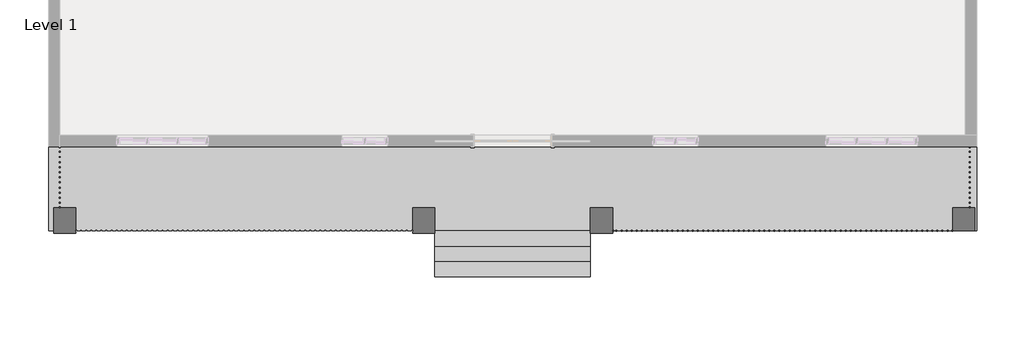
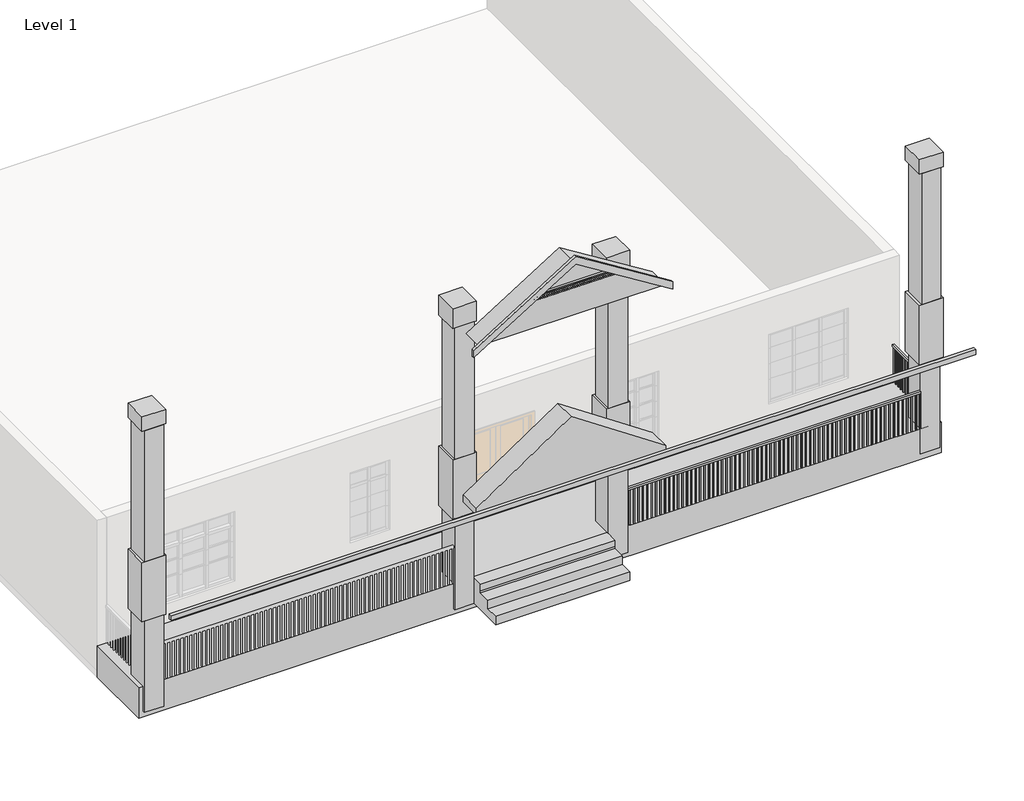
# One storey, part 3 of 3: 2 railings, 1 proxy.
"""IFC4 building model written with IfcOpenShell, lengths in millimetres."""

from ifc_helpers import new_model, si_unit, frame, origin, place, context, project, spatial, polyline, outline, extrude, transform, mapped, element, save
from components import generic_models_1_generic_models_1_befc9ee0

model = new_model("IFC4")

# Units and contexts
model_context = context("Model", 3, world=origin())
ifc_project = project(units=[si_unit("LENGTHUNIT", "METRE", prefix="MILLI")], contexts=[model_context])

# Site, building, storey
site = spatial("IfcSite", under=ifc_project)
building = spatial("IfcBuilding", under=site)
storey = spatial("IfcBuildingStorey", under=building, Name="Level 1", Elevation=0.0)

# Proxy
placement = place(None, origin())
generic_models_1_generic_models_1_shape = generic_models_1_generic_models_1_befc9ee0(model_context)
element("IfcBuildingElementProxy", 1, Name="Generic Models 1 : Generic Models 1", ObjectType="Generic Models 1 : Generic Models 1", at=placement, inside=storey, context=model_context, shape_type="MappedRepresentation", body=[
    mapped(generic_models_1_generic_models_1_shape, transform((0.0, 0.0, 0.0), x_axis=(1.0, 0.0, 0.0), y_axis=(0.0, 1.0, 0.0), z_axis=(0.0, 0.0, 1.0))),
])

# Railings
element("IfcRailing", 2, ObjectType="Handrail - Rectangular", at=placement, inside=storey, context=model_context, shape_type="SweptSolid", body=[
    extrude(outline(polyline([(8263.5579341, -8749.7902135), (8263.5579341, -8800.5902135), (1481.7579341, -8800.5902135), (1481.7579341, -8749.7902135), (8263.5579341, -8749.7902135)])), frame((0.0, 0.0, 1473.2), z_axis=(0.0, 0.0, 1.0), x_axis=(1.0, 0.0, 0.0)), (0.0, 0.0, 1.0), 50.8),
    extrude(outline(polyline([(1567.4829341, -8765.6652135), (1567.4829341, -8784.7152135), (1548.4329341, -8784.7152135), (1548.4329341, -8765.6652135), (1567.4829341, -8765.6652135)])), frame((0.0, 0.0, 609.6), z_axis=(0.0, 0.0, 1.0), x_axis=(1.0, 0.0, 0.0)), (0.0, 0.0, 1.0), 863.6),
    extrude(outline(polyline([(1669.0829341, -8765.6652135), (1669.0829341, -8784.7152135), (1650.0329341, -8784.7152135), (1650.0329341, -8765.6652135), (1669.0829341, -8765.6652135)])), frame((0.0, 0.0, 609.6), z_axis=(0.0, 0.0, 1.0), x_axis=(1.0, 0.0, 0.0)), (0.0, 0.0, 1.0), 863.6),
    extrude(outline(polyline([(1770.6829341, -8765.6652135), (1770.6829341, -8784.7152135), (1751.6329341, -8784.7152135), (1751.6329341, -8765.6652135), (1770.6829341, -8765.6652135)])), frame((0.0, 0.0, 609.6), z_axis=(0.0, 0.0, 1.0), x_axis=(1.0, 0.0, 0.0)), (0.0, 0.0, 1.0), 863.6),
    extrude(outline(polyline([(1872.2829341, -8765.6652135), (1872.2829341, -8784.7152135), (1853.2329341, -8784.7152135), (1853.2329341, -8765.6652135), (1872.2829341, -8765.6652135)])), frame((0.0, 0.0, 609.6), z_axis=(0.0, 0.0, 1.0), x_axis=(1.0, 0.0, 0.0)), (0.0, 0.0, 1.0), 863.6),
    extrude(outline(polyline([(1973.8829341, -8765.6652135), (1973.8829341, -8784.7152135), (1954.8329341, -8784.7152135), (1954.8329341, -8765.6652135), (1973.8829341, -8765.6652135)])), frame((0.0, 0.0, 609.6), z_axis=(0.0, 0.0, 1.0), x_axis=(1.0, 0.0, 0.0)), (0.0, 0.0, 1.0), 863.6),
    extrude(outline(polyline([(2075.4829341, -8765.6652135), (2075.4829341, -8784.7152135), (2056.4329341, -8784.7152135), (2056.4329341, -8765.6652135), (2075.4829341, -8765.6652135)])), frame((0.0, 0.0, 609.6), z_axis=(0.0, 0.0, 1.0), x_axis=(1.0, 0.0, 0.0)), (0.0, 0.0, 1.0), 863.6),
    extrude(outline(polyline([(2177.0829341, -8765.6652135), (2177.0829341, -8784.7152135), (2158.0329341, -8784.7152135), (2158.0329341, -8765.6652135), (2177.0829341, -8765.6652135)])), frame((0.0, 0.0, 609.6), z_axis=(0.0, 0.0, 1.0), x_axis=(1.0, 0.0, 0.0)), (0.0, 0.0, 1.0), 863.6),
    extrude(outline(polyline([(2278.6829341, -8765.6652135), (2278.6829341, -8784.7152135), (2259.6329341, -8784.7152135), (2259.6329341, -8765.6652135), (2278.6829341, -8765.6652135)])), frame((0.0, 0.0, 609.6), z_axis=(0.0, 0.0, 1.0), x_axis=(1.0, 0.0, 0.0)), (0.0, 0.0, 1.0), 863.6),
    extrude(outline(polyline([(2380.2829341, -8765.6652135), (2380.2829341, -8784.7152135), (2361.2329341, -8784.7152135), (2361.2329341, -8765.6652135), (2380.2829341, -8765.6652135)])), frame((0.0, 0.0, 609.6), z_axis=(0.0, 0.0, 1.0), x_axis=(1.0, 0.0, 0.0)), (0.0, 0.0, 1.0), 863.6),
    extrude(outline(polyline([(2481.8829341, -8765.6652135), (2481.8829341, -8784.7152135), (2462.8329341, -8784.7152135), (2462.8329341, -8765.6652135), (2481.8829341, -8765.6652135)])), frame((0.0, 0.0, 609.6), z_axis=(0.0, 0.0, 1.0), x_axis=(1.0, 0.0, 0.0)), (0.0, 0.0, 1.0), 863.6),
    extrude(outline(polyline([(2583.4829341, -8765.6652135), (2583.4829341, -8784.7152135), (2564.4329341, -8784.7152135), (2564.4329341, -8765.6652135), (2583.4829341, -8765.6652135)])), frame((0.0, 0.0, 609.6), z_axis=(0.0, 0.0, 1.0), x_axis=(1.0, 0.0, 0.0)), (0.0, 0.0, 1.0), 863.6),
    extrude(outline(polyline([(2685.0829341, -8765.6652135), (2685.0829341, -8784.7152135), (2666.0329341, -8784.7152135), (2666.0329341, -8765.6652135), (2685.0829341, -8765.6652135)])), frame((0.0, 0.0, 609.6), z_axis=(0.0, 0.0, 1.0), x_axis=(1.0, 0.0, 0.0)), (0.0, 0.0, 1.0), 863.6),
    extrude(outline(polyline([(2786.6829341, -8765.6652135), (2786.6829341, -8784.7152135), (2767.6329341, -8784.7152135), (2767.6329341, -8765.6652135), (2786.6829341, -8765.6652135)])), frame((0.0, 0.0, 609.6), z_axis=(0.0, 0.0, 1.0), x_axis=(1.0, 0.0, 0.0)), (0.0, 0.0, 1.0), 863.6),
    extrude(outline(polyline([(2888.2829341, -8765.6652135), (2888.2829341, -8784.7152135), (2869.2329341, -8784.7152135), (2869.2329341, -8765.6652135), (2888.2829341, -8765.6652135)])), frame((0.0, 0.0, 609.6), z_axis=(0.0, 0.0, 1.0), x_axis=(1.0, 0.0, 0.0)), (0.0, 0.0, 1.0), 863.6),
    extrude(outline(polyline([(2989.8829341, -8765.6652135), (2989.8829341, -8784.7152135), (2970.8329341, -8784.7152135), (2970.8329341, -8765.6652135), (2989.8829341, -8765.6652135)])), frame((0.0, 0.0, 609.6), z_axis=(0.0, 0.0, 1.0), x_axis=(1.0, 0.0, 0.0)), (0.0, 0.0, 1.0), 863.6),
    extrude(outline(polyline([(3091.4829341, -8765.6652135), (3091.4829341, -8784.7152135), (3072.4329341, -8784.7152135), (3072.4329341, -8765.6652135), (3091.4829341, -8765.6652135)])), frame((0.0, 0.0, 609.6), z_axis=(0.0, 0.0, 1.0), x_axis=(1.0, 0.0, 0.0)), (0.0, 0.0, 1.0), 863.6),
    extrude(outline(polyline([(3193.0829341, -8765.6652135), (3193.0829341, -8784.7152135), (3174.0329341, -8784.7152135), (3174.0329341, -8765.6652135), (3193.0829341, -8765.6652135)])), frame((0.0, 0.0, 609.6), z_axis=(0.0, 0.0, 1.0), x_axis=(1.0, 0.0, 0.0)), (0.0, 0.0, 1.0), 863.6),
    extrude(outline(polyline([(3294.6829341, -8765.6652135), (3294.6829341, -8784.7152135), (3275.6329341, -8784.7152135), (3275.6329341, -8765.6652135), (3294.6829341, -8765.6652135)])), frame((0.0, 0.0, 609.6), z_axis=(0.0, 0.0, 1.0), x_axis=(1.0, 0.0, 0.0)), (0.0, 0.0, 1.0), 863.6),
    extrude(outline(polyline([(3396.2829341, -8765.6652135), (3396.2829341, -8784.7152135), (3377.2329341, -8784.7152135), (3377.2329341, -8765.6652135), (3396.2829341, -8765.6652135)])), frame((0.0, 0.0, 609.6), z_axis=(0.0, 0.0, 1.0), x_axis=(1.0, 0.0, 0.0)), (0.0, 0.0, 1.0), 863.6),
    extrude(outline(polyline([(3497.8829341, -8765.6652135), (3497.8829341, -8784.7152135), (3478.8329341, -8784.7152135), (3478.8329341, -8765.6652135), (3497.8829341, -8765.6652135)])), frame((0.0, 0.0, 609.6), z_axis=(0.0, 0.0, 1.0), x_axis=(1.0, 0.0, 0.0)), (0.0, 0.0, 1.0), 863.6),
    extrude(outline(polyline([(3599.4829341, -8765.6652135), (3599.4829341, -8784.7152135), (3580.4329341, -8784.7152135), (3580.4329341, -8765.6652135), (3599.4829341, -8765.6652135)])), frame((0.0, 0.0, 609.6), z_axis=(0.0, 0.0, 1.0), x_axis=(1.0, 0.0, 0.0)), (0.0, 0.0, 1.0), 863.6),
    extrude(outline(polyline([(3701.0829341, -8765.6652135), (3701.0829341, -8784.7152135), (3682.0329341, -8784.7152135), (3682.0329341, -8765.6652135), (3701.0829341, -8765.6652135)])), frame((0.0, 0.0, 609.6), z_axis=(0.0, 0.0, 1.0), x_axis=(1.0, 0.0, 0.0)), (0.0, 0.0, 1.0), 863.6),
    extrude(outline(polyline([(3802.6829341, -8765.6652135), (3802.6829341, -8784.7152135), (3783.6329341, -8784.7152135), (3783.6329341, -8765.6652135), (3802.6829341, -8765.6652135)])), frame((0.0, 0.0, 609.6), z_axis=(0.0, 0.0, 1.0), x_axis=(1.0, 0.0, 0.0)), (0.0, 0.0, 1.0), 863.6),
    extrude(outline(polyline([(3904.2829341, -8765.6652135), (3904.2829341, -8784.7152135), (3885.2329341, -8784.7152135), (3885.2329341, -8765.6652135), (3904.2829341, -8765.6652135)])), frame((0.0, 0.0, 609.6), z_axis=(0.0, 0.0, 1.0), x_axis=(1.0, 0.0, 0.0)), (0.0, 0.0, 1.0), 863.6),
    extrude(outline(polyline([(4005.8829341, -8765.6652135), (4005.8829341, -8784.7152135), (3986.8329341, -8784.7152135), (3986.8329341, -8765.6652135), (4005.8829341, -8765.6652135)])), frame((0.0, 0.0, 609.6), z_axis=(0.0, 0.0, 1.0), x_axis=(1.0, 0.0, 0.0)), (0.0, 0.0, 1.0), 863.6),
    extrude(outline(polyline([(4107.4829341, -8765.6652135), (4107.4829341, -8784.7152135), (4088.4329341, -8784.7152135), (4088.4329341, -8765.6652135), (4107.4829341, -8765.6652135)])), frame((0.0, 0.0, 609.6), z_axis=(0.0, 0.0, 1.0), x_axis=(1.0, 0.0, 0.0)), (0.0, 0.0, 1.0), 863.6),
    extrude(outline(polyline([(4209.0829341, -8765.6652135), (4209.0829341, -8784.7152135), (4190.0329341, -8784.7152135), (4190.0329341, -8765.6652135), (4209.0829341, -8765.6652135)])), frame((0.0, 0.0, 609.6), z_axis=(0.0, 0.0, 1.0), x_axis=(1.0, 0.0, 0.0)), (0.0, 0.0, 1.0), 863.6),
    extrude(outline(polyline([(4310.6829341, -8765.6652135), (4310.6829341, -8784.7152135), (4291.6329341, -8784.7152135), (4291.6329341, -8765.6652135), (4310.6829341, -8765.6652135)])), frame((0.0, 0.0, 609.6), z_axis=(0.0, 0.0, 1.0), x_axis=(1.0, 0.0, 0.0)), (0.0, 0.0, 1.0), 863.6),
    extrude(outline(polyline([(4412.2829341, -8765.6652135), (4412.2829341, -8784.7152135), (4393.2329341, -8784.7152135), (4393.2329341, -8765.6652135), (4412.2829341, -8765.6652135)])), frame((0.0, 0.0, 609.6), z_axis=(0.0, 0.0, 1.0), x_axis=(1.0, 0.0, 0.0)), (0.0, 0.0, 1.0), 863.6),
    extrude(outline(polyline([(4513.8829341, -8765.6652135), (4513.8829341, -8784.7152135), (4494.8329341, -8784.7152135), (4494.8329341, -8765.6652135), (4513.8829341, -8765.6652135)])), frame((0.0, 0.0, 609.6), z_axis=(0.0, 0.0, 1.0), x_axis=(1.0, 0.0, 0.0)), (0.0, 0.0, 1.0), 863.6),
    extrude(outline(polyline([(4615.4829341, -8765.6652135), (4615.4829341, -8784.7152135), (4596.4329341, -8784.7152135), (4596.4329341, -8765.6652135), (4615.4829341, -8765.6652135)])), frame((0.0, 0.0, 609.6), z_axis=(0.0, 0.0, 1.0), x_axis=(1.0, 0.0, 0.0)), (0.0, 0.0, 1.0), 863.6),
    extrude(outline(polyline([(4717.0829341, -8765.6652135), (4717.0829341, -8784.7152135), (4698.0329341, -8784.7152135), (4698.0329341, -8765.6652135), (4717.0829341, -8765.6652135)])), frame((0.0, 0.0, 609.6), z_axis=(0.0, 0.0, 1.0), x_axis=(1.0, 0.0, 0.0)), (0.0, 0.0, 1.0), 863.6),
    extrude(outline(polyline([(4818.6829341, -8765.6652135), (4818.6829341, -8784.7152135), (4799.6329341, -8784.7152135), (4799.6329341, -8765.6652135), (4818.6829341, -8765.6652135)])), frame((0.0, 0.0, 609.6), z_axis=(0.0, 0.0, 1.0), x_axis=(1.0, 0.0, 0.0)), (0.0, 0.0, 1.0), 863.6),
    extrude(outline(polyline([(4920.2829341, -8765.6652135), (4920.2829341, -8784.7152135), (4901.2329341, -8784.7152135), (4901.2329341, -8765.6652135), (4920.2829341, -8765.6652135)])), frame((0.0, 0.0, 609.6), z_axis=(0.0, 0.0, 1.0), x_axis=(1.0, 0.0, 0.0)), (0.0, 0.0, 1.0), 863.6),
    extrude(outline(polyline([(5021.8829341, -8765.6652135), (5021.8829341, -8784.7152135), (5002.8329341, -8784.7152135), (5002.8329341, -8765.6652135), (5021.8829341, -8765.6652135)])), frame((0.0, 0.0, 609.6), z_axis=(0.0, 0.0, 1.0), x_axis=(1.0, 0.0, 0.0)), (0.0, 0.0, 1.0), 863.6),
    extrude(outline(polyline([(5123.4829341, -8765.6652135), (5123.4829341, -8784.7152135), (5104.4329341, -8784.7152135), (5104.4329341, -8765.6652135), (5123.4829341, -8765.6652135)])), frame((0.0, 0.0, 609.6), z_axis=(0.0, 0.0, 1.0), x_axis=(1.0, 0.0, 0.0)), (0.0, 0.0, 1.0), 863.6),
    extrude(outline(polyline([(5225.0829341, -8765.6652135), (5225.0829341, -8784.7152135), (5206.0329341, -8784.7152135), (5206.0329341, -8765.6652135), (5225.0829341, -8765.6652135)])), frame((0.0, 0.0, 609.6), z_axis=(0.0, 0.0, 1.0), x_axis=(1.0, 0.0, 0.0)), (0.0, 0.0, 1.0), 863.6),
    extrude(outline(polyline([(5326.6829341, -8765.6652135), (5326.6829341, -8784.7152135), (5307.6329341, -8784.7152135), (5307.6329341, -8765.6652135), (5326.6829341, -8765.6652135)])), frame((0.0, 0.0, 609.6), z_axis=(0.0, 0.0, 1.0), x_axis=(1.0, 0.0, 0.0)), (0.0, 0.0, 1.0), 863.6),
    extrude(outline(polyline([(5428.2829341, -8765.6652135), (5428.2829341, -8784.7152135), (5409.2329341, -8784.7152135), (5409.2329341, -8765.6652135), (5428.2829341, -8765.6652135)])), frame((0.0, 0.0, 609.6), z_axis=(0.0, 0.0, 1.0), x_axis=(1.0, 0.0, 0.0)), (0.0, 0.0, 1.0), 863.6),
    extrude(outline(polyline([(5529.8829341, -8765.6652135), (5529.8829341, -8784.7152135), (5510.8329341, -8784.7152135), (5510.8329341, -8765.6652135), (5529.8829341, -8765.6652135)])), frame((0.0, 0.0, 609.6), z_axis=(0.0, 0.0, 1.0), x_axis=(1.0, 0.0, 0.0)), (0.0, 0.0, 1.0), 863.6),
    extrude(outline(polyline([(5631.4829341, -8765.6652135), (5631.4829341, -8784.7152135), (5612.4329341, -8784.7152135), (5612.4329341, -8765.6652135), (5631.4829341, -8765.6652135)])), frame((0.0, 0.0, 609.6), z_axis=(0.0, 0.0, 1.0), x_axis=(1.0, 0.0, 0.0)), (0.0, 0.0, 1.0), 863.6),
    extrude(outline(polyline([(5733.0829341, -8765.6652135), (5733.0829341, -8784.7152135), (5714.0329341, -8784.7152135), (5714.0329341, -8765.6652135), (5733.0829341, -8765.6652135)])), frame((0.0, 0.0, 609.6), z_axis=(0.0, 0.0, 1.0), x_axis=(1.0, 0.0, 0.0)), (0.0, 0.0, 1.0), 863.6),
    extrude(outline(polyline([(5834.6829341, -8765.6652135), (5834.6829341, -8784.7152135), (5815.6329341, -8784.7152135), (5815.6329341, -8765.6652135), (5834.6829341, -8765.6652135)])), frame((0.0, 0.0, 609.6), z_axis=(0.0, 0.0, 1.0), x_axis=(1.0, 0.0, 0.0)), (0.0, 0.0, 1.0), 863.6),
    extrude(outline(polyline([(5936.2829341, -8765.6652135), (5936.2829341, -8784.7152135), (5917.2329341, -8784.7152135), (5917.2329341, -8765.6652135), (5936.2829341, -8765.6652135)])), frame((0.0, 0.0, 609.6), z_axis=(0.0, 0.0, 1.0), x_axis=(1.0, 0.0, 0.0)), (0.0, 0.0, 1.0), 863.6),
    extrude(outline(polyline([(6037.8829341, -8765.6652135), (6037.8829341, -8784.7152135), (6018.8329341, -8784.7152135), (6018.8329341, -8765.6652135), (6037.8829341, -8765.6652135)])), frame((0.0, 0.0, 609.6), z_axis=(0.0, 0.0, 1.0), x_axis=(1.0, 0.0, 0.0)), (0.0, 0.0, 1.0), 863.6),
    extrude(outline(polyline([(6139.4829341, -8765.6652135), (6139.4829341, -8784.7152135), (6120.4329341, -8784.7152135), (6120.4329341, -8765.6652135), (6139.4829341, -8765.6652135)])), frame((0.0, 0.0, 609.6), z_axis=(0.0, 0.0, 1.0), x_axis=(1.0, 0.0, 0.0)), (0.0, 0.0, 1.0), 863.6),
    extrude(outline(polyline([(6241.0829341, -8765.6652135), (6241.0829341, -8784.7152135), (6222.0329341, -8784.7152135), (6222.0329341, -8765.6652135), (6241.0829341, -8765.6652135)])), frame((0.0, 0.0, 609.6), z_axis=(0.0, 0.0, 1.0), x_axis=(1.0, 0.0, 0.0)), (0.0, 0.0, 1.0), 863.6),
    extrude(outline(polyline([(6342.6829341, -8765.6652135), (6342.6829341, -8784.7152135), (6323.6329341, -8784.7152135), (6323.6329341, -8765.6652135), (6342.6829341, -8765.6652135)])), frame((0.0, 0.0, 609.6), z_axis=(0.0, 0.0, 1.0), x_axis=(1.0, 0.0, 0.0)), (0.0, 0.0, 1.0), 863.6),
    extrude(outline(polyline([(6444.2829341, -8765.6652135), (6444.2829341, -8784.7152135), (6425.2329341, -8784.7152135), (6425.2329341, -8765.6652135), (6444.2829341, -8765.6652135)])), frame((0.0, 0.0, 609.6), z_axis=(0.0, 0.0, 1.0), x_axis=(1.0, 0.0, 0.0)), (0.0, 0.0, 1.0), 863.6),
    extrude(outline(polyline([(6545.8829341, -8765.6652135), (6545.8829341, -8784.7152135), (6526.8329341, -8784.7152135), (6526.8329341, -8765.6652135), (6545.8829341, -8765.6652135)])), frame((0.0, 0.0, 609.6), z_axis=(0.0, 0.0, 1.0), x_axis=(1.0, 0.0, 0.0)), (0.0, 0.0, 1.0), 863.6),
    extrude(outline(polyline([(6647.4829341, -8765.6652135), (6647.4829341, -8784.7152135), (6628.4329341, -8784.7152135), (6628.4329341, -8765.6652135), (6647.4829341, -8765.6652135)])), frame((0.0, 0.0, 609.6), z_axis=(0.0, 0.0, 1.0), x_axis=(1.0, 0.0, 0.0)), (0.0, 0.0, 1.0), 863.6),
    extrude(outline(polyline([(6749.0829341, -8765.6652135), (6749.0829341, -8784.7152135), (6730.0329341, -8784.7152135), (6730.0329341, -8765.6652135), (6749.0829341, -8765.6652135)])), frame((0.0, 0.0, 609.6), z_axis=(0.0, 0.0, 1.0), x_axis=(1.0, 0.0, 0.0)), (0.0, 0.0, 1.0), 863.6),
    extrude(outline(polyline([(6850.6829341, -8765.6652135), (6850.6829341, -8784.7152135), (6831.6329341, -8784.7152135), (6831.6329341, -8765.6652135), (6850.6829341, -8765.6652135)])), frame((0.0, 0.0, 609.6), z_axis=(0.0, 0.0, 1.0), x_axis=(1.0, 0.0, 0.0)), (0.0, 0.0, 1.0), 863.6),
    extrude(outline(polyline([(6952.2829341, -8765.6652135), (6952.2829341, -8784.7152135), (6933.2329341, -8784.7152135), (6933.2329341, -8765.6652135), (6952.2829341, -8765.6652135)])), frame((0.0, 0.0, 609.6), z_axis=(0.0, 0.0, 1.0), x_axis=(1.0, 0.0, 0.0)), (0.0, 0.0, 1.0), 863.6),
    extrude(outline(polyline([(7053.8829341, -8765.6652135), (7053.8829341, -8784.7152135), (7034.8329341, -8784.7152135), (7034.8329341, -8765.6652135), (7053.8829341, -8765.6652135)])), frame((0.0, 0.0, 609.6), z_axis=(0.0, 0.0, 1.0), x_axis=(1.0, 0.0, 0.0)), (0.0, 0.0, 1.0), 863.6),
    extrude(outline(polyline([(7155.4829341, -8765.6652135), (7155.4829341, -8784.7152135), (7136.4329341, -8784.7152135), (7136.4329341, -8765.6652135), (7155.4829341, -8765.6652135)])), frame((0.0, 0.0, 609.6), z_axis=(0.0, 0.0, 1.0), x_axis=(1.0, 0.0, 0.0)), (0.0, 0.0, 1.0), 863.6),
    extrude(outline(polyline([(7257.0829341, -8765.6652135), (7257.0829341, -8784.7152135), (7238.0329341, -8784.7152135), (7238.0329341, -8765.6652135), (7257.0829341, -8765.6652135)])), frame((0.0, 0.0, 609.6), z_axis=(0.0, 0.0, 1.0), x_axis=(1.0, 0.0, 0.0)), (0.0, 0.0, 1.0), 863.6),
    extrude(outline(polyline([(7358.6829341, -8765.6652135), (7358.6829341, -8784.7152135), (7339.6329341, -8784.7152135), (7339.6329341, -8765.6652135), (7358.6829341, -8765.6652135)])), frame((0.0, 0.0, 609.6), z_axis=(0.0, 0.0, 1.0), x_axis=(1.0, 0.0, 0.0)), (0.0, 0.0, 1.0), 863.6),
    extrude(outline(polyline([(7460.2829341, -8765.6652135), (7460.2829341, -8784.7152135), (7441.2329341, -8784.7152135), (7441.2329341, -8765.6652135), (7460.2829341, -8765.6652135)])), frame((0.0, 0.0, 609.6), z_axis=(0.0, 0.0, 1.0), x_axis=(1.0, 0.0, 0.0)), (0.0, 0.0, 1.0), 863.6),
    extrude(outline(polyline([(7561.8829341, -8765.6652135), (7561.8829341, -8784.7152135), (7542.8329341, -8784.7152135), (7542.8329341, -8765.6652135), (7561.8829341, -8765.6652135)])), frame((0.0, 0.0, 609.6), z_axis=(0.0, 0.0, 1.0), x_axis=(1.0, 0.0, 0.0)), (0.0, 0.0, 1.0), 863.6),
    extrude(outline(polyline([(7663.4829341, -8765.6652135), (7663.4829341, -8784.7152135), (7644.4329341, -8784.7152135), (7644.4329341, -8765.6652135), (7663.4829341, -8765.6652135)])), frame((0.0, 0.0, 609.6), z_axis=(0.0, 0.0, 1.0), x_axis=(1.0, 0.0, 0.0)), (0.0, 0.0, 1.0), 863.6),
    extrude(outline(polyline([(7765.0829341, -8765.6652135), (7765.0829341, -8784.7152135), (7746.0329341, -8784.7152135), (7746.0329341, -8765.6652135), (7765.0829341, -8765.6652135)])), frame((0.0, 0.0, 609.6), z_axis=(0.0, 0.0, 1.0), x_axis=(1.0, 0.0, 0.0)), (0.0, 0.0, 1.0), 863.6),
    extrude(outline(polyline([(7866.6829341, -8765.6652135), (7866.6829341, -8784.7152135), (7847.6329341, -8784.7152135), (7847.6329341, -8765.6652135), (7866.6829341, -8765.6652135)])), frame((0.0, 0.0, 609.6), z_axis=(0.0, 0.0, 1.0), x_axis=(1.0, 0.0, 0.0)), (0.0, 0.0, 1.0), 863.6),
    extrude(outline(polyline([(7968.2829341, -8765.6652135), (7968.2829341, -8784.7152135), (7949.2329341, -8784.7152135), (7949.2329341, -8765.6652135), (7968.2829341, -8765.6652135)])), frame((0.0, 0.0, 609.6), z_axis=(0.0, 0.0, 1.0), x_axis=(1.0, 0.0, 0.0)), (0.0, 0.0, 1.0), 863.6),
    extrude(outline(polyline([(8069.8829341, -8765.6652135), (8069.8829341, -8784.7152135), (8050.8329341, -8784.7152135), (8050.8329341, -8765.6652135), (8069.8829341, -8765.6652135)])), frame((0.0, 0.0, 609.6), z_axis=(0.0, 0.0, 1.0), x_axis=(1.0, 0.0, 0.0)), (0.0, 0.0, 1.0), 863.6),
    extrude(outline(polyline([(8171.4829341, -8765.6652135), (8171.4829341, -8784.7152135), (8152.4329341, -8784.7152135), (8152.4329341, -8765.6652135), (8171.4829341, -8765.6652135)])), frame((0.0, 0.0, 609.6), z_axis=(0.0, 0.0, 1.0), x_axis=(1.0, 0.0, 0.0)), (0.0, 0.0, 1.0), 863.6),
    extrude(outline(polyline([(1500.8079341, -8765.6652135), (1500.8079341, -8784.7152135), (1481.7579341, -8784.7152135), (1481.7579341, -8765.6652135), (1500.8079341, -8765.6652135)])), frame((0.0, 0.0, 609.6), z_axis=(0.0, 0.0, 1.0), x_axis=(1.0, 0.0, 0.0)), (0.0, 0.0, 1.0), 863.6),
    extrude(outline(polyline([(8263.5579341, -8765.6652135), (8263.5579341, -8784.7152135), (8244.5079341, -8784.7152135), (8244.5079341, -8765.6652135), (8263.5579341, -8765.6652135)])), frame((0.0, 0.0, 609.6), z_axis=(0.0, 0.0, 1.0), x_axis=(1.0, 0.0, 0.0)), (0.0, 0.0, 1.0), 863.6),
])
element("IfcRailing", 3, ObjectType="Handrail - Rectangular", at=placement, inside=storey, context=model_context, shape_type="SweptSolid", body=[
    extrude(outline(polyline([(8581.0579341, -7100.4878342), (8631.8579341, -7100.4878342), (8631.8579341, -8317.9902135), (8581.0579341, -8317.9902135), (8581.0579341, -7100.4878342)])), frame((0.0, 0.0, 1473.2), z_axis=(0.0, 0.0, 1.0), x_axis=(1.0, 0.0, 0.0)), (0.0, 0.0, 1.0), 50.8),
    extrude(outline(polyline([(8596.9329341, -8208.5628342), (8615.9829341, -8208.5628342), (8615.9829341, -8227.6128342), (8596.9329341, -8227.6128342), (8596.9329341, -8208.5628342)])), frame((0.0, 0.0, 609.6), z_axis=(0.0, 0.0, 1.0), x_axis=(1.0, 0.0, 0.0)), (0.0, 0.0, 1.0), 863.6),
    extrude(outline(polyline([(8596.9329341, -8106.9628342), (8615.9829341, -8106.9628342), (8615.9829341, -8126.0128342), (8596.9329341, -8126.0128342), (8596.9329341, -8106.9628342)])), frame((0.0, 0.0, 609.6), z_axis=(0.0, 0.0, 1.0), x_axis=(1.0, 0.0, 0.0)), (0.0, 0.0, 1.0), 863.6),
    extrude(outline(polyline([(8596.9329341, -8005.3628342), (8615.9829341, -8005.3628342), (8615.9829341, -8024.4128342), (8596.9329341, -8024.4128342), (8596.9329341, -8005.3628342)])), frame((0.0, 0.0, 609.6), z_axis=(0.0, 0.0, 1.0), x_axis=(1.0, 0.0, 0.0)), (0.0, 0.0, 1.0), 863.6),
    extrude(outline(polyline([(8596.9329341, -7903.7628342), (8615.9829341, -7903.7628342), (8615.9829341, -7922.8128342), (8596.9329341, -7922.8128342), (8596.9329341, -7903.7628342)])), frame((0.0, 0.0, 609.6), z_axis=(0.0, 0.0, 1.0), x_axis=(1.0, 0.0, 0.0)), (0.0, 0.0, 1.0), 863.6),
    extrude(outline(polyline([(8596.9329341, -7802.1628342), (8615.9829341, -7802.1628342), (8615.9829341, -7821.2128342), (8596.9329341, -7821.2128342), (8596.9329341, -7802.1628342)])), frame((0.0, 0.0, 609.6), z_axis=(0.0, 0.0, 1.0), x_axis=(1.0, 0.0, 0.0)), (0.0, 0.0, 1.0), 863.6),
    extrude(outline(polyline([(8596.9329341, -7700.5628342), (8615.9829341, -7700.5628342), (8615.9829341, -7719.6128342), (8596.9329341, -7719.6128342), (8596.9329341, -7700.5628342)])), frame((0.0, 0.0, 609.6), z_axis=(0.0, 0.0, 1.0), x_axis=(1.0, 0.0, 0.0)), (0.0, 0.0, 1.0), 863.6),
    extrude(outline(polyline([(8596.9329341, -7598.9628342), (8615.9829341, -7598.9628342), (8615.9829341, -7618.0128342), (8596.9329341, -7618.0128342), (8596.9329341, -7598.9628342)])), frame((0.0, 0.0, 609.6), z_axis=(0.0, 0.0, 1.0), x_axis=(1.0, 0.0, 0.0)), (0.0, 0.0, 1.0), 863.6),
    extrude(outline(polyline([(8596.9329341, -7497.3628342), (8615.9829341, -7497.3628342), (8615.9829341, -7516.4128342), (8596.9329341, -7516.4128342), (8596.9329341, -7497.3628342)])), frame((0.0, 0.0, 609.6), z_axis=(0.0, 0.0, 1.0), x_axis=(1.0, 0.0, 0.0)), (0.0, 0.0, 1.0), 863.6),
    extrude(outline(polyline([(8596.9329341, -7395.7628342), (8615.9829341, -7395.7628342), (8615.9829341, -7414.8128342), (8596.9329341, -7414.8128342), (8596.9329341, -7395.7628342)])), frame((0.0, 0.0, 609.6), z_axis=(0.0, 0.0, 1.0), x_axis=(1.0, 0.0, 0.0)), (0.0, 0.0, 1.0), 863.6),
    extrude(outline(polyline([(8596.9329341, -7294.1628342), (8615.9829341, -7294.1628342), (8615.9829341, -7313.2128342), (8596.9329341, -7313.2128342), (8596.9329341, -7294.1628342)])), frame((0.0, 0.0, 609.6), z_axis=(0.0, 0.0, 1.0), x_axis=(1.0, 0.0, 0.0)), (0.0, 0.0, 1.0), 863.6),
    extrude(outline(polyline([(8596.9329341, -7192.5628342), (8615.9829341, -7192.5628342), (8615.9829341, -7211.6128342), (8596.9329341, -7211.6128342), (8596.9329341, -7192.5628342)])), frame((0.0, 0.0, 609.6), z_axis=(0.0, 0.0, 1.0), x_axis=(1.0, 0.0, 0.0)), (0.0, 0.0, 1.0), 863.6),
    extrude(outline(polyline([(8596.9329341, -8298.9402135), (8615.9829341, -8298.9402135), (8615.9829341, -8317.9902135), (8596.9329341, -8317.9902135), (8596.9329341, -8298.9402135)])), frame((0.0, 0.0, 609.6), z_axis=(0.0, 0.0, 1.0), x_axis=(1.0, 0.0, 0.0)), (0.0, 0.0, 1.0), 863.6),
    extrude(outline(polyline([(8596.9329341, -7100.4878342), (8615.9829341, -7100.4878342), (8615.9829341, -7119.5378342), (8596.9329341, -7119.5378342), (8596.9329341, -7100.4878342)])), frame((0.0, 0.0, 609.6), z_axis=(0.0, 0.0, 1.0), x_axis=(1.0, 0.0, 0.0)), (0.0, 0.0, 1.0), 863.6),
])

save(model, "model.ifc")

# Revit data of these elements
# Type "Handrail - Rectangular"
#   Assembly Code = "C2010400"
#   built-in parameter 1008612 = 0.0416667 (stored number, unit not read)
#   built-in parameter 1008611 = 0.0416667 (stored number, unit not read)
#   built-in parameter 1008609 = 0.333333 (stored number, unit not read)
#   built-in parameter 1008604 = 0.166667 (stored number, unit not read)
#   built-in parameter 1008603 = 0.166667 (stored number, unit not read)
#   Railing Height = 3' - 0"
#   built-in parameter 1008630 = 2
#   built-in parameter 1008610 = 2
#   built-in parameter 1008618 = Baluster - Square : 3/4"
# Element 1 (IfcBuildingElementProxy, "Generic Models 1 : Generic Models 1")
#   Phase Created = New Construction
#   Materials on its faces: "Gravel", "Laminate, Ivory, Matte", "wood pier", "Gypsum Wall Board", "wood wall"
# Elements 2, 3 (IfcRailing, "Handrail - Rectangular")
#   built-in parameter 1008621 = 2 (stored number, unit not read)
#   Phase Created = New Construction
# Materials
#   "Gravel": class "Generic", colour RGB 120 120 120, transparency 0, Description = "Crushed stone or gravel", Cost = 0
#   "Laminate, Ivory, Matte": class "Plastic", colour RGB 247 247 239, transparency 0, Description = "Plastic Laminate - Ivory, Matte", Cost = 0
#   "wood pier": class "Generic", colour RGB 120 120 120, transparency 0, Cost = 0
#   "Gypsum Wall Board": class "Generic", colour RGB 127 127 127, transparency 0, Description = "Gypsum Wall Board", Cost = 0
#   "wood wall": class "Generic", colour RGB 120 120 120, transparency 0, Cost = 0
